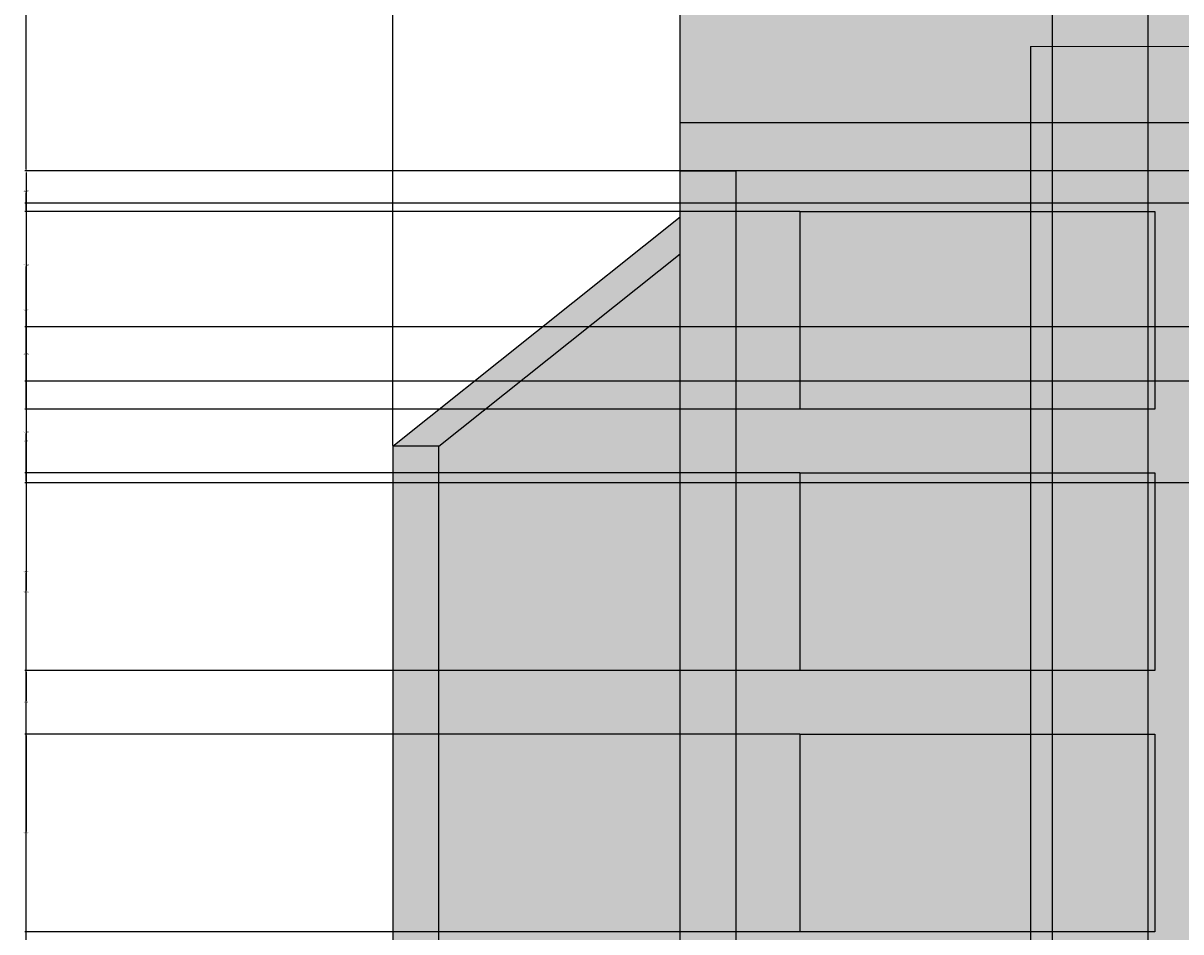
# Model space of a CAD drawing. Units: inches. Extents: x 3024 to 4744, y 1110 to 2100.
# Tile 2 of 29: x 3024 to 3168, y 1181 to 1294. Entities that reach past the tile are written whole.
import ezdxf

# ---------------------------------------------------------------- set-up
doc = ezdxf.new("R2010")
doc.units = ezdxf.units.IN
for name, color, linetype, lineweight in [('A-ANNO-DIMS', 2, 'Continuous', 18), ('A-ELEV', 7, 'Continuous', 25), ('A-ELEV-PATT', 252, 'Continuous', 13), ('A-GLAZ', 4, 'Continuous', 18)]:
    doc.layers.add(name, color=color, linetype=linetype, lineweight=lineweight)
doc.styles.get("Standard").update_dxf_attribs({"font": 'arial.ttf'})
doc.dimstyles.get("Standard").update_dxf_attribs({"dimtxt": 0.18, "dimasz": 0.18, "dimexe": 0.18, "dimexo": 0.0625, "dimgap": 0.09, "dimtad": 0, "dimtih": 1, "dimtoh": 1, "dimdec": 1, "dimzin": 0, "dimdsep": 46, "dimlunit": 3, "dimtxsty": 'Standard', "dimcen": 0.09, "dimadec": 0, "dimazin": 0, "dimtfac": 1, "dimtdec": 1, "dimtofl": 0, "dimtmove": 0, "dimatfit": 3, "dimfxl": 1, "dimtolj": 1, "dimtzin": 0, "dimarcsym": 0})

# ---------------------------------------------------------------- blocks, each defined once
blk = doc.blocks.new('WIN-BALCONY-A')
for p, q in [((3169.4, 1897.49), (3148.97, 1897.49)), ((3169.4, 1897.49), (3148.97, 1897.49)), ((3169.4, 1897.49), (3292.61, 1897.49)), ((3169.4, 1897.49), (3292.61, 1897.49)), ((3169.4, 1795.04), (3148.97, 1795.04)), ((3169.4, 1795.04), (3148.97, 1795.04)), ((3169.4, 1795.04), (3292.61, 1795.04)), ((3169.4, 1795.04), (3292.61, 1795.04))]:
    blk.add_line(p, q)
for points in [[(3148.97, 1897.49), (3148.97, 1905.61), (3292.61, 1905.61), (3292.61, 1897.49)], [(3148.97, 1897.49), (3148.97, 1905.61), (3292.61, 1905.61), (3292.61, 1897.49)], [(3292.61, 1795.04), (3292.61, 1785.61), (3148.97, 1785.61), (3148.97, 1795.04)], [(3292.61, 1795.04), (3292.61, 1785.61), (3148.97, 1785.61), (3148.97, 1795.04)]]:
    blk.add_lwpolyline(points)
for points in [[(3154.33, 1806.87), (3160.86, 1806.87), (3160.86, 1897.49), (3154.33, 1897.49)], [(3154.33, 1806.87), (3160.86, 1806.87), (3160.86, 1897.49), (3154.33, 1897.49)], [(3272.18, 1795.04), (3169.4, 1795.04), (3169.4, 1897.49), (3272.18, 1897.49)], [(3272.18, 1795.04), (3169.4, 1795.04), (3169.4, 1897.49), (3272.18, 1897.49)], [(3287.25, 1806.87), (3280.72, 1806.87), (3280.72, 1897.49), (3287.25, 1897.49)], [(3287.25, 1806.87), (3280.72, 1806.87), (3280.72, 1897.49), (3287.25, 1897.49)], [(3268.18, 1799.04), (3173.4, 1799.04), (3173.4, 1893.49), (3268.18, 1893.49)], [(3268.18, 1799.04), (3173.4, 1799.04), (3173.4, 1893.49), (3268.18, 1893.49)], [(3220.05, 1893.49), (3221.52, 1893.49), (3221.52, 1799.04), (3220.05, 1799.04)], [(3220.05, 1893.49), (3221.52, 1893.49), (3221.52, 1799.04), (3220.05, 1799.04)], [(3163.53, 1795.04), (3151.66, 1795.04), (3151.66, 1806.87), (3163.53, 1806.87)], [(3163.53, 1795.04), (3151.66, 1795.04), (3151.66, 1806.87), (3163.53, 1806.87)], [(3276.51, 1795.04), (3288.38, 1795.04), (3288.38, 1806.87), (3276.51, 1806.87)], [(3276.51, 1795.04), (3288.38, 1795.04), (3288.38, 1806.87), (3276.51, 1806.87)]]:
    blk.add_lwpolyline(points, close=True)
blk = doc.blocks.new('*D51')
at = {"layer": 'A-ANNO-DIMS', "color": 0, "lineweight": -2, "transparency": 16777216}
for p, q in [((3148.97, 1290.98), (3148.97, 1109.93)), ((3105.47, 1155.55), (3105.47, 1109.93)), ((3105.65, 1110.11), (3126.89, 1110.11)), ((3148.79, 1110.11), (3127.55, 1110.11))]:
    blk.add_line(p, q, dxfattribs=at)
at = {"layer": 'A-ANNO-DIMS', "color": 0, "transparency": 16777216}
for points in [[(3105.65, 1110.14), (3105.65, 1110.08), (3105.47, 1110.11)], [(3148.79, 1110.14), (3148.79, 1110.08), (3148.97, 1110.11)]]:
    blk.add_solid(points, dxfattribs=at)
at = {"layer": 'Defpoints', "color": 0, "transparency": 16777216}
for p in [(3148.97, 1291.04), (3105.47, 1155.61), (3148.97, 1110.11)]:
    blk.add_point(p, dxfattribs=at)
at = {"layer": 'A-ANNO-DIMS', "color": 0, "transparency": 16777216, "insert": (3127.22, 1110.11), "char_height": 0.18, "attachment_point": 5}
blk.add_mtext('\\A1;43.5', dxfattribs=at)
blk = doc.blocks.new('*D52')
at = {"layer": 'A-ANNO-DIMS', "color": 0, "lineweight": -2, "transparency": 16777216}
for p, q in [((3148.97, 1290.98), (3148.97, 1109.93)), ((3170.16, 1170.96), (3170.16, 1109.93)), ((3149.15, 1110.11), (3159.17, 1110.11)), ((3169.98, 1110.11), (3159.96, 1110.11))]:
    blk.add_line(p, q, dxfattribs=at)
at = {"layer": 'A-ANNO-DIMS', "color": 0, "transparency": 16777216}
for points in [[(3149.15, 1110.14), (3149.15, 1110.08), (3148.97, 1110.11)], [(3169.98, 1110.14), (3169.98, 1110.08), (3170.16, 1110.11)]]:
    blk.add_solid(points, dxfattribs=at)
at = {"layer": 'Defpoints', "color": 0, "transparency": 16777216}
for p in [(3148.97, 1291.04), (3170.16, 1171.02), (3170.16, 1110.11)]:
    blk.add_point(p, dxfattribs=at)
at = {"layer": 'A-ANNO-DIMS', "color": 0, "transparency": 16777216, "insert": (3159.57, 1110.11), "char_height": 0.18, "attachment_point": 5}
blk.add_mtext('\\A1;21.19', dxfattribs=at)
blk = doc.blocks.new('*D64')
at = {"layer": 'A-ANNO-DIMS', "color": 0, "lineweight": -2, "transparency": 16777216}
for p, q in [((3069.79, 1241.5), (3069.79, 2100.44)), ((3069.97, 2100.26), (3405.08, 2100.26)), ((3740.97, 2100.26), (3405.87, 2100.26)), ((3741.15, 1241.5), (3741.15, 2100.44))]:
    blk.add_line(p, q, dxfattribs=at)
at = {"layer": 'A-ANNO-DIMS', "color": 0, "transparency": 16777216}
for points in [[(3069.97, 2100.29), (3069.97, 2100.23), (3069.79, 2100.26)], [(3740.97, 2100.29), (3740.97, 2100.23), (3741.15, 2100.26)]]:
    blk.add_solid(points, dxfattribs=at)
at = {"layer": 'Defpoints', "color": 0, "transparency": 16777216}
for p in [(3741.15, 2100.26), (3069.79, 1241.43), (3741.15, 1241.43)]:
    blk.add_point(p, dxfattribs=at)
at = {"layer": 'A-ANNO-DIMS', "color": 0, "transparency": 16777216, "insert": (3405.47, 2100.26), "char_height": 0.18, "attachment_point": 5}
blk.add_mtext('\\A1;671.4', dxfattribs=at)
blk = doc.blocks.new('*D66')
at = {"layer": 'A-ANNO-DIMS', "color": 0, "lineweight": -2, "transparency": 16777216}
for p, q in [((3105.41, 1275.61), (3024.11, 1275.61)), ((3024.29, 1275.43), (3024.29, 1223.5)), ((3024.29, 1171.2), (3024.29, 1223.14)), ((3105.41, 1171.02), (3024.11, 1171.02))]:
    blk.add_line(p, q, dxfattribs=at)
at = {"layer": 'A-ANNO-DIMS', "color": 0, "transparency": 16777216}
for points in [[(3024.26, 1275.43), (3024.32, 1275.43), (3024.29, 1275.61)], [(3024.26, 1171.2), (3024.32, 1171.2), (3024.29, 1171.02)]]:
    blk.add_solid(points, dxfattribs=at)
at = {"layer": 'Defpoints', "color": 0, "transparency": 16777216}
for p in [(3024.29, 1275.61), (3105.47, 1275.61), (3105.47, 1171.02)]:
    blk.add_point(p, dxfattribs=at)
at = {"layer": 'A-ANNO-DIMS', "color": 0, "transparency": 16777216, "insert": (3024.29, 1223.32), "char_height": 0.18, "attachment_point": 5}
blk.add_mtext('\\A1;104.59', dxfattribs=at)
blk = doc.blocks.new('*D67')
at = {"layer": 'A-ANNO-DIMS', "color": 0, "lineweight": -2, "transparency": 16777216}
for p, q in [((3105.41, 1401.61), (3024.11, 1401.61)), ((3024.29, 1401.43), (3024.29, 1338.79)), ((3024.29, 1275.79), (3024.29, 1338.43)), ((3105.41, 1275.61), (3024.11, 1275.61))]:
    blk.add_line(p, q, dxfattribs=at)
at = {"layer": 'A-ANNO-DIMS', "color": 0, "transparency": 16777216}
for points in [[(3024.26, 1401.43), (3024.32, 1401.43), (3024.29, 1401.61)], [(3024.26, 1275.79), (3024.32, 1275.79), (3024.29, 1275.61)]]:
    blk.add_solid(points, dxfattribs=at)
at = {"layer": 'Defpoints', "color": 0, "transparency": 16777216}
for p in [(3024.29, 1401.61), (3105.47, 1401.61), (3105.47, 1275.61)]:
    blk.add_point(p, dxfattribs=at)
at = {"layer": 'A-ANNO-DIMS', "color": 0, "transparency": 16777216, "insert": (3024.29, 1338.61), "char_height": 0.18, "attachment_point": 5}
blk.add_mtext('\\A1;126', dxfattribs=at)
blk = doc.blocks.new('*D89')
at = {"layer": 'A-ANNO-DIMS', "color": 0, "lineweight": -2, "transparency": 16777216}
for p, q in [((3151.66, 1794.98), (3151.66, 1109.93)), ((3163.53, 1794.98), (3163.53, 1109.93)), ((3151.84, 1110.11), (3157.14, 1110.11)), ((3163.35, 1110.11), (3158.05, 1110.11))]:
    blk.add_line(p, q, dxfattribs=at)
at = {"layer": 'A-ANNO-DIMS', "color": 0, "transparency": 16777216}
for points in [[(3151.84, 1110.14), (3151.84, 1110.08), (3151.66, 1110.11)], [(3163.35, 1110.14), (3163.35, 1110.08), (3163.53, 1110.11)]]:
    blk.add_solid(points, dxfattribs=at)
at = {"layer": 'Defpoints', "color": 0, "transparency": 16777216}
for p in [(3151.66, 1795.04), (3163.53, 1795.04), (3163.53, 1110.11)]:
    blk.add_point(p, dxfattribs=at)
at = {"layer": 'A-ANNO-DIMS', "color": 0, "transparency": 16777216, "insert": (3157.59, 1110.11), "char_height": 0.18, "attachment_point": 5}
blk.add_mtext('\\A1;11.866', dxfattribs=at)
blk = doc.blocks.new('*D114')
at = {"layer": 'A-ANNO-DIMS', "color": 0, "lineweight": -2, "transparency": 16777216}
for p, q in [((3120.31, 1205.67), (3024.11, 1205.67)), ((3024.29, 1205.49), (3024.29, 1193.58)), ((3024.29, 1181.3), (3024.29, 1193.22)), ((3120.31, 1181.12), (3024.11, 1181.12))]:
    blk.add_line(p, q, dxfattribs=at)
at = {"layer": 'A-ANNO-DIMS', "color": 0, "transparency": 16777216}
for points in [[(3024.26, 1205.49), (3024.32, 1205.49), (3024.29, 1205.67)], [(3024.26, 1181.3), (3024.32, 1181.3), (3024.29, 1181.12)]]:
    blk.add_solid(points, dxfattribs=at)
at = {"layer": 'Defpoints', "color": 0, "transparency": 16777216}
for p in [(3024.29, 1205.67), (3120.37, 1205.67), (3120.37, 1181.12)]:
    blk.add_point(p, dxfattribs=at)
at = {"layer": 'A-ANNO-DIMS', "color": 0, "transparency": 16777216, "insert": (3024.29, 1193.4), "char_height": 0.18, "attachment_point": 5}
blk.add_mtext('\\A1;24.55', dxfattribs=at)
blk = doc.blocks.new('*D115')
at = {"layer": 'A-ANNO-DIMS', "color": 0, "lineweight": -2, "transparency": 16777216}
for p, q in [((3120.31, 1213.57), (3024.11, 1213.57)), ((3024.29, 1213.39), (3024.29, 1209.8)), ((3024.29, 1205.85), (3024.29, 1209.44)), ((3120.31, 1205.67), (3024.11, 1205.67))]:
    blk.add_line(p, q, dxfattribs=at)
at = {"layer": 'A-ANNO-DIMS', "color": 0, "transparency": 16777216}
for points in [[(3024.26, 1213.39), (3024.32, 1213.39), (3024.29, 1213.57)], [(3024.26, 1205.85), (3024.32, 1205.85), (3024.29, 1205.67)]]:
    blk.add_solid(points, dxfattribs=at)
at = {"layer": 'Defpoints', "color": 0, "transparency": 16777216}
for p in [(3024.29, 1213.57), (3120.37, 1213.57), (3120.37, 1205.67)]:
    blk.add_point(p, dxfattribs=at)
at = {"layer": 'A-ANNO-DIMS', "color": 0, "transparency": 16777216, "insert": (3024.29, 1209.62), "char_height": 0.18, "attachment_point": 5}
blk.add_mtext('\\A1;7.898', dxfattribs=at)
blk = doc.blocks.new('*D116')
at = {"layer": 'A-ANNO-DIMS', "color": 0, "lineweight": -2, "transparency": 16777216}
for p, q in [((3120.31, 1238.12), (3024.11, 1238.12)), ((3024.29, 1237.94), (3024.29, 1226.03)), ((3024.29, 1213.75), (3024.29, 1225.66)), ((3120.31, 1213.57), (3024.11, 1213.57))]:
    blk.add_line(p, q, dxfattribs=at)
at = {"layer": 'A-ANNO-DIMS', "color": 0, "transparency": 16777216}
for points in [[(3024.26, 1237.94), (3024.32, 1237.94), (3024.29, 1238.12)], [(3024.26, 1213.75), (3024.32, 1213.75), (3024.29, 1213.57)]]:
    blk.add_solid(points, dxfattribs=at)
at = {"layer": 'Defpoints', "color": 0, "transparency": 16777216}
for p in [(3024.29, 1238.12), (3120.37, 1238.12), (3120.37, 1213.57)]:
    blk.add_point(p, dxfattribs=at)
at = {"layer": 'A-ANNO-DIMS', "color": 0, "transparency": 16777216, "insert": (3024.29, 1225.84), "char_height": 0.18, "attachment_point": 5}
blk.add_mtext('\\A1;24.55', dxfattribs=at)
blk = doc.blocks.new('*D117')
at = {"layer": 'A-ANNO-DIMS', "color": 0, "lineweight": -2, "transparency": 16777216}
for p, q in [((3120.31, 1246.02), (3024.11, 1246.02)), ((3024.29, 1245.84), (3024.29, 1242.25)), ((3024.29, 1238.3), (3024.29, 1241.89)), ((3120.31, 1238.12), (3024.11, 1238.12))]:
    blk.add_line(p, q, dxfattribs=at)
at = {"layer": 'A-ANNO-DIMS', "color": 0, "transparency": 16777216}
for points in [[(3024.26, 1245.84), (3024.32, 1245.84), (3024.29, 1246.02)], [(3024.26, 1238.3), (3024.32, 1238.3), (3024.29, 1238.12)]]:
    blk.add_solid(points, dxfattribs=at)
at = {"layer": 'Defpoints', "color": 0, "transparency": 16777216}
for p in [(3024.29, 1246.02), (3120.37, 1246.02), (3120.37, 1238.12)]:
    blk.add_point(p, dxfattribs=at)
at = {"layer": 'A-ANNO-DIMS', "color": 0, "transparency": 16777216, "insert": (3024.29, 1242.07), "char_height": 0.18, "attachment_point": 5}
blk.add_mtext('\\A1;7.898', dxfattribs=at)
blk = doc.blocks.new('*D118')
at = {"layer": 'A-ANNO-DIMS', "color": 0, "lineweight": -2, "transparency": 16777216}
for p, q in [((3120.31, 1270.56), (3024.11, 1270.56)), ((3024.29, 1270.38), (3024.29, 1258.47)), ((3024.29, 1246.2), (3024.29, 1258.11)), ((3120.31, 1246.02), (3024.11, 1246.02))]:
    blk.add_line(p, q, dxfattribs=at)
at = {"layer": 'A-ANNO-DIMS', "color": 0, "transparency": 16777216}
for points in [[(3024.26, 1270.38), (3024.32, 1270.38), (3024.29, 1270.56)], [(3024.26, 1246.2), (3024.32, 1246.2), (3024.29, 1246.02)]]:
    blk.add_solid(points, dxfattribs=at)
at = {"layer": 'Defpoints', "color": 0, "transparency": 16777216}
for p in [(3024.29, 1270.56), (3120.37, 1270.56), (3120.37, 1246.02)]:
    blk.add_point(p, dxfattribs=at)
at = {"layer": 'A-ANNO-DIMS', "color": 0, "transparency": 16777216, "insert": (3024.29, 1258.29), "char_height": 0.18, "attachment_point": 5}
blk.add_mtext('\\A1;24.55', dxfattribs=at)
blk = doc.blocks.new('*D119')
at = {"layer": 'A-ANNO-DIMS', "color": 0, "lineweight": -2, "transparency": 16777216}
for p, q in [((3112.32, 1275.61), (3024.11, 1275.61)), ((3024.29, 1275.43), (3024.29, 1273.27)), ((3024.29, 1270.74), (3024.29, 1272.91)), ((3120.31, 1270.56), (3024.11, 1270.56))]:
    blk.add_line(p, q, dxfattribs=at)
at = {"layer": 'A-ANNO-DIMS', "color": 0, "transparency": 16777216}
for points in [[(3024.26, 1275.43), (3024.32, 1275.43), (3024.29, 1275.61)], [(3024.26, 1270.74), (3024.32, 1270.74), (3024.29, 1270.56)]]:
    blk.add_solid(points, dxfattribs=at)
at = {"layer": 'Defpoints', "color": 0, "transparency": 16777216}
for p in [(3024.29, 1275.61), (3112.38, 1275.61), (3120.37, 1270.56)]:
    blk.add_point(p, dxfattribs=at)
at = {"layer": 'A-ANNO-DIMS', "color": 0, "transparency": 16777216, "insert": (3024.29, 1273.09), "char_height": 0.18, "attachment_point": 5}
blk.add_mtext('\\A1;5.047', dxfattribs=at)
blk = doc.blocks.new('*D127')
at = {"layer": 'A-ANNO-DIMS', "color": 0, "lineweight": -2, "transparency": 16777216}
for p, q in [((3174.1, 1271.61), (3024.11, 1271.61)), ((3024.29, 1271.43), (3024.29, 1264.1)), ((3024.29, 1256.41), (3024.29, 1263.74)), ((3188.2, 1256.23), (3024.11, 1256.23))]:
    blk.add_line(p, q, dxfattribs=at)
at = {"layer": 'A-ANNO-DIMS', "color": 0, "transparency": 16777216}
for points in [[(3024.26, 1271.43), (3024.32, 1271.43), (3024.29, 1271.61)], [(3024.26, 1256.41), (3024.32, 1256.41), (3024.29, 1256.23)]]:
    blk.add_solid(points, dxfattribs=at)
at = {"layer": 'Defpoints', "color": 0, "transparency": 16777216}
for p in [(3174.16, 1271.61), (3024.29, 1256.23), (3188.26, 1256.23)]:
    blk.add_point(p, dxfattribs=at)
at = {"layer": 'A-ANNO-DIMS', "color": 0, "transparency": 16777216, "insert": (3024.29, 1263.92), "char_height": 0.18, "attachment_point": 5}
blk.add_mtext('\\A1;15.384', dxfattribs=at)
blk = doc.blocks.new('*D128')
at = {"layer": 'A-ANNO-DIMS', "color": 0, "lineweight": -2, "transparency": 16777216}
for p, q in [((3188.2, 1256.23), (3024.11, 1256.23)), ((3024.29, 1256.05), (3024.29, 1253.04)), ((3024.29, 1249.67), (3024.29, 1252.68)), ((3188.2, 1249.49), (3024.11, 1249.49))]:
    blk.add_line(p, q, dxfattribs=at)
at = {"layer": 'A-ANNO-DIMS', "color": 0, "transparency": 16777216}
for points in [[(3024.26, 1256.05), (3024.32, 1256.05), (3024.29, 1256.23)], [(3024.26, 1249.67), (3024.32, 1249.67), (3024.29, 1249.49)]]:
    blk.add_solid(points, dxfattribs=at)
at = {"layer": 'Defpoints', "color": 0, "transparency": 16777216}
for p in [(3188.26, 1256.23), (3024.29, 1249.49), (3188.26, 1249.49)]:
    blk.add_point(p, dxfattribs=at)
at = {"layer": 'A-ANNO-DIMS', "color": 0, "transparency": 16777216, "insert": (3024.29, 1252.86), "char_height": 0.18, "attachment_point": 5}
blk.add_mtext('\\A1;6.738', dxfattribs=at)
blk = doc.blocks.new('*D129')
at = {"layer": 'A-ANNO-DIMS', "color": 0, "lineweight": -2, "transparency": 16777216}
for p, q in [((3188.2, 1249.49), (3024.11, 1249.49)), ((3024.29, 1249.31), (3024.29, 1243.37)), ((3024.29, 1237.07), (3024.29, 1243.01)), ((3188.2, 1236.89), (3024.11, 1236.89))]:
    blk.add_line(p, q, dxfattribs=at)
at = {"layer": 'A-ANNO-DIMS', "color": 0, "transparency": 16777216}
for points in [[(3024.26, 1249.31), (3024.32, 1249.31), (3024.29, 1249.49)], [(3024.26, 1237.07), (3024.32, 1237.07), (3024.29, 1236.89)]]:
    blk.add_solid(points, dxfattribs=at)
at = {"layer": 'Defpoints', "color": 0, "transparency": 16777216}
for p in [(3188.26, 1249.49), (3024.29, 1236.89), (3188.26, 1236.89)]:
    blk.add_point(p, dxfattribs=at)
at = {"layer": 'A-ANNO-DIMS', "color": 0, "transparency": 16777216, "insert": (3024.29, 1243.19), "char_height": 0.18, "attachment_point": 5}
blk.add_mtext('\\A1;12.603', dxfattribs=at)

msp = doc.modelspace()

# ---------------------------------------------------------------- hatches: boundary and pattern name
at = {"layer": 'A-ELEV-PATT'}
h = msp.add_hatch(color=256, dxfattribs=at)
h.dxf.hatch_style = 1
h.paths.add_polyline_path([(3491.8271, 2054.7584), (3320.5658, 2054.7584), (3320.5658, 2043.5286), (3491.8271, 2043.5286)])
h.paths.add_polyline_path([(3292.6051, 1905.6112), (3148.9694, 1905.6112), (3148.9694, 1897.4879), (3169.3964, 1897.4879), (3292.6051, 1897.4879)])
h.paths.add_polyline_path([(3292.6051, 1795.0431), (3169.3964, 1795.0431), (3148.9694, 1795.0431), (3148.9694, 1785.6112), (3292.6051, 1785.6112)])
h.paths.add_polyline_path([(3292.6051, 1779.6112), (3148.9694, 1779.6112), (3148.9694, 1771.4879), (3169.3964, 1771.4879), (3292.6051, 1771.4879)])
h.paths.add_polyline_path([(3292.6051, 1669.0431), (3169.3964, 1669.0431), (3148.9694, 1669.0431), (3148.9694, 1659.6112), (3292.6051, 1659.6112)])
h.paths.add_polyline_path([(3292.6051, 1653.6112), (3148.9694, 1653.6112), (3148.9694, 1645.4879), (3169.3964, 1645.4879), (3292.6051, 1645.4879)])
h.paths.add_polyline_path([(3292.6051, 1543.0431), (3169.3964, 1543.0431), (3148.9694, 1543.0431), (3148.9694, 1533.6112), (3292.6051, 1533.6112)])
h.paths.add_polyline_path([(3292.6051, 1527.6112), (3148.9694, 1527.6112), (3148.9694, 1519.4879), (3169.3964, 1519.4879), (3292.6051, 1519.4879)])
h.paths.add_polyline_path([(3292.6051, 1401.6112), (3148.9694, 1401.6112), (3148.9694, 1393.4879), (3169.3964, 1393.4879), (3292.6051, 1393.4879)])
h.paths.add_polyline_path([(3292.6051, 1417.0431), (3169.3964, 1417.0431), (3148.9694, 1417.0431), (3148.9694, 1407.6112), (3292.6051, 1407.6112)])
h.paths.add_polyline_path([(3292.6051, 1291.0431), (3169.3964, 1291.0431), (3148.9694, 1291.0431), (3148.9694, 1281.6112), (3292.6051, 1281.6112)])
h.paths.add_polyline_path([(3654.037, 1165.0431), (3530.8283, 1165.0431), (3510.4013, 1165.0431), (3510.4013, 1155.6112), (3654.037, 1155.6112)])
h.paths.add_polyline_path([(3654.037, 1275.6112), (3510.4013, 1275.6112), (3510.4013, 1267.4879), (3530.8283, 1267.4879), (3654.037, 1267.4879)])
h.paths.add_polyline_path([(3654.037, 1291.0431), (3530.8283, 1291.0431), (3510.4013, 1291.0431), (3510.4013, 1281.6112), (3654.037, 1281.6112)])
h.paths.add_polyline_path([(3654.037, 1417.0431), (3530.8283, 1417.0431), (3510.4013, 1417.0431), (3510.4013, 1407.6112), (3654.037, 1407.6112)])
h.paths.add_polyline_path([(3654.037, 1401.6112), (3510.4013, 1401.6112), (3510.4013, 1393.4879), (3530.8283, 1393.4879), (3654.037, 1393.4879)])
h.paths.add_polyline_path([(3654.037, 1543.0431), (3530.8283, 1543.0431), (3510.4013, 1543.0431), (3510.4013, 1533.6112), (3654.037, 1533.6112)])
h.paths.add_polyline_path([(3654.037, 1527.6112), (3510.4013, 1527.6112), (3510.4013, 1519.4879), (3530.8283, 1519.4879), (3654.037, 1519.4879)])
h.paths.add_polyline_path([(3654.037, 1653.6112), (3510.4013, 1653.6112), (3510.4013, 1645.4879), (3530.8283, 1645.4879), (3654.037, 1645.4879)])
h.paths.add_polyline_path([(3654.037, 1669.0431), (3530.8283, 1669.0431), (3510.4013, 1669.0431), (3510.4013, 1659.6112), (3654.037, 1659.6112)])
h.paths.add_polyline_path([(3654.037, 1779.6112), (3510.4013, 1779.6112), (3510.4013, 1771.4879), (3530.8283, 1771.4879), (3654.037, 1771.4879)])
h.paths.add_polyline_path([(3654.037, 1795.0431), (3530.8283, 1795.0431), (3510.4013, 1795.0431), (3510.4013, 1785.6112), (3654.037, 1785.6112)])
h.paths.add_polyline_path([(3654.037, 1905.6112), (3510.4013, 1905.6112), (3510.4013, 1897.4879), (3530.8283, 1897.4879), (3654.037, 1897.4879)])
h = msp.add_hatch(color=256, dxfattribs=at)
h.dxf.hatch_style = 1
h.paths.add_polyline_path([(3329.7033, 1407.6112), (3105.4722, 1407.6112), (3105.4722, 1401.6112), (3329.7033, 1401.6112)])
h.paths.add_polyline_path([(3329.7033, 1281.6112), (3105.4722, 1281.6112), (3105.4722, 1275.6112), (3112.3838, 1275.6112), (3329.7033, 1275.6112)])
h.paths.add_polyline_path([(3329.7033, 1533.6112), (3105.4722, 1533.6112), (3105.4722, 1527.6112), (3329.7033, 1527.6112)])
h.paths.add_polyline_path([(3329.7033, 1659.6112), (3105.4722, 1659.6112), (3105.4722, 1653.6112), (3329.7033, 1653.6112)])
h.paths.add_polyline_path([(3329.7033, 1785.6112), (3105.4722, 1785.6112), (3105.4722, 1779.6112), (3329.7033, 1779.6112)])
h.paths.add_polyline_path([(3329.7033, 1911.6112), (3105.4722, 1911.6112), (3095.7158, 1911.6112), (3095.7158, 1905.6112), (3329.7033, 1905.6112)])
h.paths.add_polyline_path([(3715.2286, 1911.6112), (3705.4722, 1911.6112), (3705.4722, 1905.6112), (3715.2286, 1905.6112)])
h.paths.add_polyline_path([(3688.5588, 1911.6112), (3481.2411, 1911.6112), (3481.2411, 1905.6112), (3688.5588, 1905.6112)])
h = msp.add_hatch(color=256, dxfattribs=at)
h.dxf.hatch_style = 1
h.paths.add_polyline_path([(3154.3287, 1897.4879), (3148.9694, 1897.4879), (3148.9694, 1905.6112), (3105.4722, 1905.6112), (3105.4722, 1785.6112), (3148.9694, 1785.6112), (3148.9694, 1795.0431), (3151.6604, 1795.0431), (3151.6604, 1806.8674), (3154.3287, 1806.8674)])
h.paths.add_polyline_path([(3329.7033, 1905.6112), (3292.6051, 1905.6112), (3292.6051, 1897.4879), (3287.2458, 1897.4879), (3287.2458, 1806.8674), (3288.3759, 1806.8674), (3288.3759, 1795.0431), (3292.6051, 1795.0431), (3292.6051, 1785.6112), (3329.7033, 1785.6112)])
h.paths.add_polyline_path([(3154.3287, 1771.4879), (3148.9694, 1771.4879), (3148.9694, 1779.6112), (3105.4722, 1779.6112), (3105.4722, 1659.6112), (3148.9694, 1659.6112), (3148.9694, 1669.0431), (3151.6604, 1669.0431), (3151.6604, 1680.8674), (3154.3287, 1680.8674)])
h.paths.add_polyline_path([(3329.7033, 1779.6112), (3292.6051, 1779.6112), (3292.6051, 1771.4879), (3287.2458, 1771.4879), (3287.2458, 1680.8674), (3288.3759, 1680.8674), (3288.3759, 1669.0431), (3292.6051, 1669.0431), (3292.6051, 1659.6112), (3329.7033, 1659.6112)])
h.paths.add_polyline_path([(3154.3287, 1645.4879), (3148.9694, 1645.4879), (3148.9694, 1653.6112), (3105.4722, 1653.6112), (3105.4722, 1533.6112), (3148.9694, 1533.6112), (3148.9694, 1543.0431), (3151.6604, 1543.0431), (3151.6604, 1554.8674), (3154.3287, 1554.8674)])
h.paths.add_polyline_path([(3329.7033, 1653.6112), (3292.6051, 1653.6112), (3292.6051, 1645.4879), (3287.2458, 1645.4879), (3287.2458, 1554.8674), (3288.3759, 1554.8674), (3288.3759, 1543.0431), (3292.6051, 1543.0431), (3292.6051, 1533.6112), (3329.7033, 1533.6112)])
h.paths.add_polyline_path([(3329.7033, 1527.6112), (3292.6051, 1527.6112), (3292.6051, 1519.4879), (3287.2458, 1519.4879), (3287.2458, 1428.8674), (3288.3759, 1428.8674), (3288.3759, 1417.0431), (3292.6051, 1417.0431), (3292.6051, 1407.6112), (3329.7033, 1407.6112)])
h.paths.add_polyline_path([(3329.7033, 1401.6112), (3292.6051, 1401.6112), (3292.6051, 1393.4879), (3287.2458, 1393.4879), (3287.2458, 1302.8674), (3288.3759, 1302.8674), (3288.3759, 1291.0431), (3292.6051, 1291.0431), (3292.6051, 1281.6112), (3329.7033, 1281.6112)])
h.paths.add_polyline_path([(3154.3287, 1393.4879), (3148.9694, 1393.4879), (3148.9694, 1401.6112), (3105.4722, 1401.6112), (3105.4722, 1281.6112), (3148.9694, 1281.6112), (3148.9694, 1291.0431), (3151.6604, 1291.0431), (3151.6604, 1302.8674), (3154.3287, 1302.8674)])
h.paths.add_polyline_path([(3154.3287, 1519.4879), (3148.9694, 1519.4879), (3148.9694, 1527.6112), (3105.4722, 1527.6112), (3105.4722, 1407.6112), (3148.9694, 1407.6112), (3148.9694, 1417.0431), (3151.6604, 1417.0431), (3151.6604, 1428.8674), (3154.3287, 1428.8674)])
h.paths.add_polyline_path([(3515.7606, 1897.4879), (3510.4013, 1897.4879), (3510.4013, 1905.6112), (3481.2411, 1905.6112), (3481.2411, 1785.6112), (3510.4013, 1785.6112), (3510.4013, 1795.0431), (3513.0923, 1795.0431), (3513.0923, 1806.8674), (3515.7606, 1806.8674)])
h.paths.add_polyline_path([(3688.5588, 1905.6112), (3654.037, 1905.6112), (3654.037, 1897.4879), (3648.6777, 1897.4879), (3648.6777, 1806.8674), (3649.8078, 1806.8674), (3649.8078, 1795.0431), (3654.037, 1795.0431), (3654.037, 1785.6112), (3688.5588, 1785.6112)])
h.paths.add_polyline_path([(3515.7606, 1771.4879), (3510.4013, 1771.4879), (3510.4013, 1779.6112), (3481.2411, 1779.6112), (3481.2411, 1659.6112), (3510.4013, 1659.6112), (3510.4013, 1669.0431), (3513.0923, 1669.0431), (3513.0923, 1680.8674), (3515.7606, 1680.8674)])
h.paths.add_polyline_path([(3688.5588, 1779.6112), (3654.037, 1779.6112), (3654.037, 1771.4879), (3648.6777, 1771.4879), (3648.6777, 1680.8674), (3649.8078, 1680.8674), (3649.8078, 1669.0431), (3654.037, 1669.0431), (3654.037, 1659.6112), (3688.5588, 1659.6112)])
h.paths.add_polyline_path([(3515.7606, 1645.4879), (3510.4013, 1645.4879), (3510.4013, 1653.6112), (3481.2411, 1653.6112), (3481.2411, 1533.6112), (3510.4013, 1533.6112), (3510.4013, 1543.0431), (3513.0923, 1543.0431), (3513.0923, 1554.8674), (3515.7606, 1554.8674)])
h.paths.add_polyline_path([(3688.5588, 1653.6112), (3654.037, 1653.6112), (3654.037, 1645.4879), (3648.6777, 1645.4879), (3648.6777, 1554.8674), (3649.8078, 1554.8674), (3649.8078, 1543.0431), (3654.037, 1543.0431), (3654.037, 1533.6112), (3688.5588, 1533.6112)])
h.paths.add_polyline_path([(3515.7606, 1519.4879), (3510.4013, 1519.4879), (3510.4013, 1527.6112), (3481.2411, 1527.6112), (3481.2411, 1407.6112), (3510.4013, 1407.6112), (3510.4013, 1417.0431), (3513.0923, 1417.0431), (3513.0923, 1428.8674), (3515.7606, 1428.8674)])
h.paths.add_polyline_path([(3688.5588, 1527.6112), (3654.037, 1527.6112), (3654.037, 1519.4879), (3648.6777, 1519.4879), (3648.6777, 1428.8674), (3649.8078, 1428.8674), (3649.8078, 1417.0431), (3654.037, 1417.0431), (3654.037, 1407.6112), (3688.5588, 1407.6112)])
h.paths.add_polyline_path([(3515.7606, 1393.4879), (3510.4013, 1393.4879), (3510.4013, 1401.6112), (3481.2411, 1401.6112), (3481.2411, 1281.6112), (3510.4013, 1281.6112), (3510.4013, 1291.0431), (3513.0923, 1291.0431), (3513.0923, 1302.8674), (3515.7606, 1302.8674)])
h.paths.add_polyline_path([(3688.5588, 1401.6112), (3654.037, 1401.6112), (3654.037, 1393.4879), (3648.6777, 1393.4879), (3648.6777, 1302.8674), (3649.8078, 1302.8674), (3649.8078, 1291.0431), (3654.037, 1291.0431), (3654.037, 1281.6112), (3688.5588, 1281.6112)])
h.paths.add_polyline_path([(3515.7606, 1267.4879), (3510.4013, 1267.4879), (3510.4013, 1275.6112), (3481.2411, 1275.6112), (3481.2411, 1155.6112), (3510.4013, 1155.6112), (3510.4013, 1165.0431), (3513.0923, 1165.0431), (3513.0923, 1176.8674), (3515.7606, 1176.8674)])
h.paths.add_polyline_path([(3688.5588, 1275.6112), (3654.037, 1275.6112), (3654.037, 1267.4879), (3648.6777, 1267.4879), (3648.6777, 1176.8674), (3649.8078, 1176.8674), (3649.8078, 1165.0431), (3654.037, 1165.0431), (3654.037, 1155.6112), (3688.5588, 1155.6112)])
h.paths.add_polyline_path([(3112.3838, 1275.6112), (3105.4722, 1275.6112), (3105.4722, 1171.0239), (3112.3838, 1171.0239)])
h = msp.add_hatch(color=256, dxfattribs=at)
h.dxf.hatch_style = 1
h.paths.add_polyline_path([(3169.3964, 1897.4879), (3160.8586, 1897.4879), (3160.8586, 1806.8674), (3163.5269, 1806.8674), (3163.5269, 1795.0431), (3169.3964, 1795.0431)])
h.paths.add_polyline_path([(3280.716, 1897.4879), (3272.1781, 1897.4879), (3272.1781, 1795.0431), (3276.5094, 1795.0431), (3276.5094, 1806.8674), (3280.716, 1806.8674)])
h.paths.add_polyline_path([(3280.716, 1771.4879), (3272.1781, 1771.4879), (3272.1781, 1669.0431), (3276.5094, 1669.0431), (3276.5094, 1680.8674), (3280.716, 1680.8674)])
h.paths.add_polyline_path([(3169.3964, 1771.4879), (3160.8586, 1771.4879), (3160.8586, 1680.8674), (3163.5269, 1680.8674), (3163.5269, 1669.0431), (3169.3964, 1669.0431)])
h.paths.add_polyline_path([(3169.3964, 1645.4879), (3160.8586, 1645.4879), (3160.8586, 1554.8674), (3163.5269, 1554.8674), (3163.5269, 1543.0431), (3169.3964, 1543.0431)])
h.paths.add_polyline_path([(3280.716, 1645.4879), (3272.1781, 1645.4879), (3272.1781, 1543.0431), (3276.5094, 1543.0431), (3276.5094, 1554.8674), (3280.716, 1554.8674)])
h.paths.add_polyline_path([(3169.3964, 1519.4879), (3160.8586, 1519.4879), (3160.8586, 1428.8674), (3163.5269, 1428.8674), (3163.5269, 1417.0431), (3169.3964, 1417.0431)])
h.paths.add_polyline_path([(3280.716, 1519.4879), (3272.1781, 1519.4879), (3272.1781, 1417.0431), (3276.5094, 1417.0431), (3276.5094, 1428.8674), (3280.716, 1428.8674)])
h.paths.add_polyline_path([(3169.3964, 1393.4879), (3160.8586, 1393.4879), (3160.8586, 1302.8674), (3163.5269, 1302.8674), (3163.5269, 1291.0431), (3169.3964, 1291.0431)])
h.paths.add_polyline_path([(3280.716, 1393.4879), (3272.1781, 1393.4879), (3272.1781, 1291.0431), (3276.5094, 1291.0431), (3276.5094, 1302.8674), (3280.716, 1302.8674)])
h.paths.add_polyline_path([(3642.1479, 1267.4879), (3633.61, 1267.4879), (3633.61, 1165.0431), (3637.9413, 1165.0431), (3637.9413, 1176.8674), (3642.1479, 1176.8674)])
h.paths.add_polyline_path([(3530.8283, 1267.4879), (3522.2905, 1267.4879), (3522.2905, 1176.8674), (3524.9588, 1176.8674), (3524.9588, 1165.0431), (3530.8283, 1165.0431)])
h.paths.add_polyline_path([(3642.1479, 1393.4879), (3633.61, 1393.4879), (3633.61, 1291.0431), (3637.9413, 1291.0431), (3637.9413, 1302.8674), (3642.1479, 1302.8674)])
h.paths.add_polyline_path([(3530.8283, 1393.4879), (3522.2905, 1393.4879), (3522.2905, 1302.8674), (3524.9588, 1302.8674), (3524.9588, 1291.0431), (3530.8283, 1291.0431)])
h.paths.add_polyline_path([(3530.8283, 1519.4879), (3522.2905, 1519.4879), (3522.2905, 1428.8674), (3524.9588, 1428.8674), (3524.9588, 1417.0431), (3530.8283, 1417.0431)])
h.paths.add_polyline_path([(3642.1479, 1519.4879), (3633.61, 1519.4879), (3633.61, 1417.0431), (3637.9413, 1417.0431), (3637.9413, 1428.8674), (3642.1479, 1428.8674)])
h.paths.add_polyline_path([(3530.8283, 1645.4879), (3522.2905, 1645.4879), (3522.2905, 1554.8674), (3524.9588, 1554.8674), (3524.9588, 1543.0431), (3530.8283, 1543.0431)])
h.paths.add_polyline_path([(3642.1479, 1645.4879), (3633.61, 1645.4879), (3633.61, 1543.0431), (3637.9413, 1543.0431), (3637.9413, 1554.8674), (3642.1479, 1554.8674)])
h.paths.add_polyline_path([(3642.1479, 1771.4879), (3633.61, 1771.4879), (3633.61, 1669.0431), (3637.9413, 1669.0431), (3637.9413, 1680.8674), (3642.1479, 1680.8674)])
h.paths.add_polyline_path([(3530.8283, 1771.4879), (3522.2905, 1771.4879), (3522.2905, 1680.8674), (3524.9588, 1680.8674), (3524.9588, 1669.0431), (3530.8283, 1669.0431)])
h.paths.add_polyline_path([(3530.8283, 1897.4879), (3522.2905, 1897.4879), (3522.2905, 1806.8674), (3524.9588, 1806.8674), (3524.9588, 1795.0431), (3530.8283, 1795.0431)])
h.paths.add_polyline_path([(3642.1479, 1897.4879), (3633.61, 1897.4879), (3633.61, 1795.0431), (3637.9413, 1795.0431), (3637.9413, 1806.8674), (3642.1479, 1806.8674)])
h = msp.add_hatch(color=256, dxfattribs=at)
h.dxf.hatch_style = 1
h.paths.add_polyline_path([(3163.5269, 1302.8674), (3151.6604, 1302.8674), (3151.6604, 1291.0431), (3163.5269, 1291.0431)])
h.paths.add_polyline_path([(3288.3759, 1302.8674), (3276.5094, 1302.8674), (3276.5094, 1291.0431), (3288.3759, 1291.0431)])
h.paths.add_polyline_path([(3288.3759, 1428.8674), (3276.5094, 1428.8674), (3276.5094, 1417.0431), (3288.3759, 1417.0431)])
h.paths.add_polyline_path([(3163.5269, 1428.8674), (3151.6604, 1428.8674), (3151.6604, 1417.0431), (3163.5269, 1417.0431)])
h.paths.add_polyline_path([(3163.5269, 1554.8674), (3151.6604, 1554.8674), (3151.6604, 1543.0431), (3163.5269, 1543.0431)])
h.paths.add_polyline_path([(3288.3759, 1554.8674), (3276.5094, 1554.8674), (3276.5094, 1543.0431), (3288.3759, 1543.0431)])
h.paths.add_polyline_path([(3163.5269, 1680.8674), (3151.6604, 1680.8674), (3151.6604, 1669.0431), (3163.5269, 1669.0431)])
h.paths.add_polyline_path([(3288.3759, 1680.8674), (3276.5094, 1680.8674), (3276.5094, 1669.0431), (3288.3759, 1669.0431)])
h.paths.add_polyline_path([(3163.5269, 1806.8674), (3151.6604, 1806.8674), (3151.6604, 1795.0431), (3163.5269, 1795.0431)])
h.paths.add_polyline_path([(3288.3759, 1806.8674), (3276.5094, 1806.8674), (3276.5094, 1795.0431), (3288.3759, 1795.0431)])
h.paths.add_polyline_path([(3524.9588, 1806.8674), (3513.0923, 1806.8674), (3513.0923, 1795.0431), (3524.9588, 1795.0431)])
h.paths.add_polyline_path([(3649.8078, 1806.8674), (3637.9413, 1806.8674), (3637.9413, 1795.0431), (3649.8078, 1795.0431)])
h.paths.add_polyline_path([(3524.9588, 1680.8674), (3513.0923, 1680.8674), (3513.0923, 1669.0431), (3524.9588, 1669.0431)])
h.paths.add_polyline_path([(3649.8078, 1680.8674), (3637.9413, 1680.8674), (3637.9413, 1669.0431), (3649.8078, 1669.0431)])
h.paths.add_polyline_path([(3524.9588, 1554.8674), (3513.0923, 1554.8674), (3513.0923, 1543.0431), (3524.9588, 1543.0431)])
h.paths.add_polyline_path([(3649.8078, 1554.8674), (3637.9413, 1554.8674), (3637.9413, 1543.0431), (3649.8078, 1543.0431)])
h.paths.add_polyline_path([(3524.9588, 1428.8674), (3513.0923, 1428.8674), (3513.0923, 1417.0431), (3524.9588, 1417.0431)])
h.paths.add_polyline_path([(3649.8078, 1428.8674), (3637.9413, 1428.8674), (3637.9413, 1417.0431), (3649.8078, 1417.0431)])
h.paths.add_polyline_path([(3524.9588, 1302.8674), (3513.0923, 1302.8674), (3513.0923, 1291.0431), (3524.9588, 1291.0431)])
h.paths.add_polyline_path([(3649.8078, 1302.8674), (3637.9413, 1302.8674), (3637.9413, 1291.0431), (3649.8078, 1291.0431)])
h.paths.add_polyline_path([(3524.9588, 1176.8674), (3513.0923, 1176.8674), (3513.0923, 1165.0431), (3524.9588, 1165.0431)])
h.paths.add_polyline_path([(3649.8078, 1176.8674), (3637.9413, 1176.8674), (3637.9413, 1165.0431), (3649.8078, 1165.0431)])
h = msp.add_hatch(color=256, dxfattribs=at)
h.dxf.hatch_style = 1
h.paths.add_polyline_path([(3329.7033, 1275.6112), (3274.3877, 1275.6112), (3274.3877, 1171.0239), (3329.7033, 1171.0239)])
h.paths.add_polyline_path([(3323.3693, 1246.0161), (3279.3584, 1246.0161), (3279.3584, 1270.5642), (3323.3693, 1270.5642)], flags=16)
h.paths.add_polyline_path([(3323.3693, 1238.118), (3323.3693, 1213.5699), (3279.3584, 1213.5699), (3279.3584, 1238.118)], flags=16)
h.paths.add_polyline_path([(3323.3693, 1205.6718), (3323.3693, 1181.1236), (3279.3584, 1181.1236), (3279.3584, 1205.6718)], flags=16)
h.paths.add_polyline_path([(3170.1608, 1275.6112), (3112.3838, 1275.6112), (3112.3838, 1171.0239), (3118.1176, 1171.0239), (3170.1608, 1171.0239)])
h.paths.add_polyline_path([(3120.3696, 1246.0161), (3120.3696, 1270.5642), (3164.3806, 1270.5642), (3164.3806, 1246.0161)], flags=16)
h.paths.add_polyline_path([(3120.3696, 1238.118), (3164.3806, 1238.118), (3164.3806, 1213.5699), (3120.3696, 1213.5699)], flags=16)
h.paths.add_polyline_path([(3120.3696, 1205.6718), (3164.3806, 1205.6718), (3164.3806, 1181.1236), (3120.3696, 1181.1236)], flags=16)
h = msp.add_hatch(color=256, dxfattribs=at)
h.dxf.hatch_style = 1
h.paths.add_polyline_path([(3323.3693, 1270.5642), (3279.3584, 1270.5642), (3279.3584, 1246.0161), (3323.3693, 1246.0161)])
h.paths.add_polyline_path([(3323.3693, 1238.118), (3279.3584, 1238.118), (3279.3584, 1213.5699), (3323.3693, 1213.5699)])
h.paths.add_polyline_path([(3323.3693, 1205.6718), (3279.3584, 1205.6718), (3279.3584, 1181.1236), (3323.3693, 1181.1236)])
h.paths.add_polyline_path([(3164.3806, 1270.5642), (3120.3696, 1270.5642), (3120.3696, 1246.0161), (3164.3806, 1246.0161)])
h.paths.add_polyline_path([(3164.3806, 1238.118), (3120.3696, 1238.118), (3120.3696, 1213.5699), (3164.3806, 1213.5699)])
h.paths.add_polyline_path([(3164.3806, 1205.6718), (3120.3696, 1205.6718), (3120.3696, 1181.1236), (3164.3806, 1181.1236)])
h = msp.add_hatch(color=256, dxfattribs=at)
h.dxf.hatch_style = 1
h.paths.add_polyline_path([(3329.7033, 1171.0239), (3256.7794, 1171.0239, -0.21182003), (3255.8005, 1171.0239), (3249.6327, 1171.0239, -0.21182003), (3248.6539, 1171.0239), (3195.8947, 1171.0239, -0.21182003), (3194.9159, 1171.0239), (3188.7481, 1171.0239, -0.21182003), (3187.7692, 1171.0239), (3118.1176, 1171.0239), (3115.5754, 1168.0828), (3115.5754, 1155.6112), (3329.7033, 1155.6112)])
h.paths.add_polyline_path([(3101.9647, 1168.0828), (3103.2358, 1169.5534), (3069.7937, 1169.5534), (3069.7937, 1155.6112), (3101.9647, 1155.6112)])
h.paths.add_polyline_path([(3115.5754, 1168.0828), (3101.9647, 1168.0828), (3101.9647, 1155.6112), (3105.4722, 1155.6112), (3115.5754, 1155.6112)])
h.paths.add_polyline_path([(3118.1176, 1171.0239), (3104.5069, 1171.0239), (3101.9647, 1168.0828), (3115.5754, 1168.0828)])
h.paths.add_polyline_path([(3105.4722, 1265.3254), (3075.5369, 1241.4341), (3075.5369, 1169.5534), (3103.2358, 1169.5534), (3104.5069, 1171.0239), (3105.4722, 1171.0239)])
h.paths.add_polyline_path([(3105.4722, 1265.3254), (3105.4722, 1269.9091), (3069.7937, 1241.4341), (3075.5369, 1241.4341)])
h.paths.add_polyline_path([(3075.5369, 1241.4341), (3069.7937, 1241.4341), (3069.7937, 1169.5534), (3075.5369, 1169.5534)])
h.paths.add_polyline_path([(3735.4075, 1241.4341), (3705.4722, 1265.3254), (3705.4722, 1169.5534), (3735.4075, 1169.5534)])
h.paths.add_polyline_path([(3705.4722, 1269.9091), (3705.4722, 1265.3254), (3735.4075, 1241.4341), (3741.1507, 1241.4341)])
h.paths.add_polyline_path([(3741.1507, 1241.4341), (3735.4075, 1241.4341), (3735.4075, 1169.5534), (3741.1507, 1169.5534)])
h.paths.add_polyline_path([(3741.1507, 1169.5534), (3735.4075, 1169.5534), (3705.4722, 1169.5534), (3705.4722, 1155.6112), (3741.1507, 1155.6112)])
h = msp.add_hatch(dxfattribs=at)
h.set_pattern_fill('AR-B816', color=256, scale=0.01)
h.paths.add_polyline_path([(3105.4722, 1265.3254), (3075.5369, 1241.4341), (3075.5369, 1169.5534), (3103.2358, 1169.5534), (3104.5069, 1171.0239), (3105.4722, 1171.0239)])
h.paths.add_polyline_path([(3105.4722, 1265.3254), (3105.4722, 1269.9091), (3069.7937, 1241.4341), (3075.5369, 1241.4341)])
h.paths.add_polyline_path([(3075.5369, 1241.4341), (3069.7937, 1241.4341), (3069.7937, 1169.5534), (3075.5369, 1169.5534)])
h.paths.add_polyline_path([(3735.4075, 1241.4341), (3705.4722, 1265.3254), (3705.4722, 1169.5534), (3735.4075, 1169.5534)])
h.paths.add_polyline_path([(3705.4722, 1269.9091), (3705.4722, 1265.3254), (3735.4075, 1241.4341), (3741.1507, 1241.4341)])
h.paths.add_polyline_path([(3741.1507, 1241.4341), (3735.4075, 1241.4341), (3735.4075, 1169.5534), (3741.1507, 1169.5534)])

# ---------------------------------------------------------------- linework, layer by layer
at = {"layer": 'A-ELEV'}
for p, q in [((3105.4722, 1171.0239), (3105.4722, 1905.6112)), ((3105.4722, 1171.0239), (3105.4722, 1905.6112)), ((3105.4722, 1275.6112), (3105.4722, 1281.6112)), ((3105.4722, 1281.6112), (3329.7033, 1281.6112)), ((3105.4722, 1275.6112), (3105.4722, 1281.6112)), ((3105.4722, 1281.6112), (3329.7033, 1281.6112)), ((3329.7033, 1275.6112), (3105.4722, 1275.6112)), ((3329.7033, 1275.6112), (3105.4722, 1275.6112)), ((3069.7937, 1241.4341), (3105.4722, 1269.9091)), ((3069.7937, 1241.4341), (3105.4722, 1269.9091)), ((3075.5369, 1241.4341), (3105.4722, 1265.3254)), ((3075.5369, 1241.4341), (3105.4722, 1265.3254))]:
    msp.add_line(p, q, dxfattribs=at)
msp.add_lwpolyline([(3105.4722, 1275.6112), (3112.3838, 1275.6112), (3112.3838, 1171.0239)], dxfattribs=at)
msp.add_lwpolyline([(3105.4722, 1275.6112), (3112.3838, 1275.6112), (3112.3838, 1171.0239)], dxfattribs=at)
for points in [[(3120.3696, 1270.5642), (3164.3806, 1270.5642), (3164.3806, 1246.0161), (3120.3696, 1246.0161)], [(3069.7937, 1169.5534), (3075.5369, 1169.5534), (3075.5369, 1241.4341), (3069.7937, 1241.4341)], [(3069.7937, 1169.5534), (3075.5369, 1169.5534), (3075.5369, 1241.4341), (3069.7937, 1241.4341)], [(3120.3696, 1238.118), (3164.3806, 1238.118), (3164.3806, 1213.5699), (3120.3696, 1213.5699)], [(3120.3696, 1205.6718), (3164.3806, 1205.6718), (3164.3806, 1181.1236), (3120.3696, 1181.1236)]]:
    msp.add_lwpolyline(points, close=True, dxfattribs=at)

# ---------------------------------------------------------------- block references
at = {"layer": 'A-GLAZ'}
msp.add_blockref('WIN-BALCONY-A', (0, -504), dxfattribs=at)

# ---------------------------------------------------------------- dimensions: what is measured, and where the dimension line sits
at = {"layer": 'A-ANNO-DIMS'}
for base, p1, p2, override, picture, middle in [((3741.1507, 2100.2584), (3069.7937, 1241.4341), (3741.1507, 1241.4341), {"dimdec": 1, "dimlfac": 1, "dimrnd": 0, "dimzin": 0, "dimdsep": 46, "dimlunit": 2}, '*D64', (3405.4722, 2100.2584)), ((3163.526875, 1110.111173), (3151.660378, 1795.043127), (3163.526875, 1795.043127), {"dimdec": 3, "dimlfac": 1, "dimrnd": 0, "dimzin": 0, "dimdsep": 46, "dimlunit": 2}, '*D89', (3157.593627, 1110.111173)), ((3148.9694, 1110.1112), (3105.4722, 1155.6112), (3148.9694, 1291.0431), {"dimdec": 1, "dimlfac": 1, "dimrnd": 0, "dimzin": 0, "dimdsep": 46, "dimlunit": 2}, '*D51', (3127.2208, 1110.1112)), ((3170.1608, 1110.1112), (3148.9694, 1291.0431), (3170.1608, 1171.0239), {"dimdec": 2, "dimlfac": 1, "dimrnd": 0, "dimzin": 0, "dimdsep": 46, "dimlunit": 2}, '*D52', (3159.5651, 1110.1112))]:
    dim = msp.add_linear_dim(base=base, p1=p1, p2=p2, dimstyle='Standard', override=override, dxfattribs=at)
    dim.commit()
    dim.dimension.update_dxf_attribs({"geometry": picture, "text_midpoint": middle})
for base, p1, p2, override, picture, middle in [((3024.2937, 1401.6112), (3105.4722, 1275.6112), (3105.4722, 1401.6112), {"dimdec": 0, "dimlfac": 1, "dimrnd": 0, "dimzin": 0, "dimdsep": 46, "dimlunit": 2}, '*D67', (3024.2937, 1338.6112)), ((3024.2937, 1275.6112), (3105.4722, 1171.0239), (3105.4722, 1275.6112), {"dimdec": 2, "dimlfac": 1, "dimrnd": 0, "dimzin": 0, "dimdsep": 46, "dimlunit": 2}, '*D66', (3024.2937, 1223.3176)), ((3024.2937, 1275.6112), (3120.3696, 1270.5642), (3112.3838, 1275.6112), {"dimdec": 3, "dimlfac": 1, "dimrnd": 0, "dimzin": 0, "dimdsep": 46, "dimlunit": 2}, '*D119', (3024.2937, 1273.0877)), ((3024.2937, 1256.2276), (3174.1608, 1271.6112), (3188.2586, 1256.2276), {"dimdec": 3, "dimlfac": 1, "dimrnd": 0, "dimzin": 0, "dimdsep": 46, "dimlunit": 2}, '*D127', (3024.2937, 1263.9194)), ((3024.2937, 1270.5642), (3120.3696, 1246.0161), (3120.3696, 1270.5642), {"dimdec": 2, "dimlfac": 1, "dimrnd": 0, "dimzin": 0, "dimdsep": 46, "dimlunit": 2}, '*D118', (3024.2937, 1258.2901)), ((3024.2937, 1249.4899), (3188.2586, 1256.2276), (3188.2586, 1249.4899), {"dimdec": 3, "dimlfac": 1, "dimrnd": 0, "dimzin": 0, "dimdsep": 46, "dimlunit": 2}, '*D128', (3024.2937, 1252.8587)), ((3024.2937, 1236.8869), (3188.2586, 1249.4899), (3188.2586, 1236.8869), {"dimdec": 3, "dimlfac": 1, "dimrnd": 0, "dimzin": 0, "dimdsep": 46, "dimlunit": 2}, '*D129', (3024.2937, 1243.1884)), ((3024.2937, 1246.0161), (3120.3696, 1238.118), (3120.3696, 1246.0161), {"dimdec": 3, "dimlfac": 1, "dimrnd": 0, "dimzin": 0, "dimdsep": 46, "dimlunit": 2}, '*D117', (3024.2937, 1242.067)), ((3024.2937, 1238.118), (3120.3696, 1213.5699), (3120.3696, 1238.118), {"dimdec": 2, "dimlfac": 1, "dimrnd": 0, "dimzin": 0, "dimdsep": 46, "dimlunit": 2}, '*D116', (3024.2937, 1225.8439)), ((3024.2937, 1213.5699), (3120.3696, 1205.6718), (3120.3696, 1213.5699), {"dimdec": 3, "dimlfac": 1, "dimrnd": 0, "dimzin": 0, "dimdsep": 46, "dimlunit": 2}, '*D115', (3024.2937, 1209.6208)), ((3024.2937, 1205.6718), (3120.3696, 1181.1236), (3120.3696, 1205.6718), {"dimdec": 2, "dimlfac": 1, "dimrnd": 0, "dimzin": 0, "dimdsep": 46, "dimlunit": 2}, '*D114', (3024.2937, 1193.3977))]:
    dim = msp.add_linear_dim(base=base, p1=p1, p2=p2, angle=90, dimstyle='Standard', override=override, dxfattribs=at)
    dim.commit()
    dim.dimension.update_dxf_attribs({"geometry": picture, "text_midpoint": middle})

doc.saveas('drawing.dxf')
